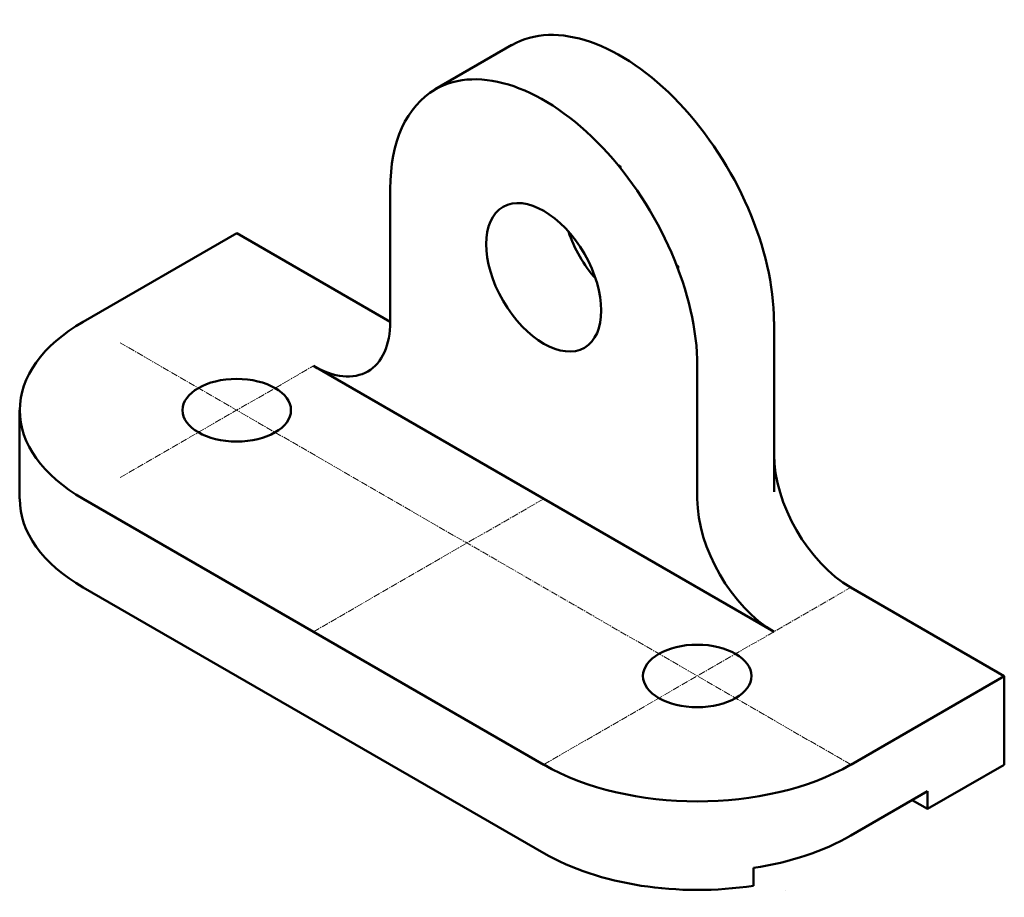
# Model space of a CAD drawing. Units: millimetres. Extents: x -15 to 96, y 7 to 106.
import ezdxf

# ---------------------------------------------------------------- set-up
doc = ezdxf.new("R2010")
doc.units = ezdxf.units.MM
doc.header["$MEASUREMENT"] = 0
doc.linetypes.add('CENTER2', pattern=[1.125, 0.75, -0.125, 0.125, -0.125])
doc.layers.add('M-CNTR', color=1, linetype='CENTER2', lineweight=18)
doc.layers.add('M-OUTL', color=7, linetype='Continuous', lineweight=50)

msp = doc.modelspace()

# ---------------------------------------------------------------- linework, layer by layer
at = {"layer": 'M-CNTR'}
for p, q in [((78.96, 21.51), (-3.47, 69.1)), ((-3.47, 53.92), (18.33, 66.51)), ((18.33, 36.51), (44.31, 51.51)), ((44.31, 21.51), (79.06, 41.57))]:
    msp.add_line(p, q, dxfattribs=at)
at = {"layer": 'M-OUTL'}
for p, q in [((40.73, 102.73), (32.07, 97.73)), ((27, 71.5), (27, 86.5)), ((-7.64, 71.5), (9.68, 81.5)), ((27, 71.5), (9.68, 81.5)), ((70.3, 71.51), (70.3, 52.29)), ((70.3, 36.5), (18.34, 66.5)), ((61.64, 66.5), (61.64, 51.5)), ((-14.82, 51.5), (-14.82, 61.5)), ((44.32, 21.5), (-7.64, 51.5)), ((44.32, 11.5), (-7.64, 41.5)), ((96.28, 31.5), (78.96, 41.5)), ((78.96, 21.5), (96.28, 31.5)), ((96.28, 21.5), (96.28, 31.5)), ((87.62, 16.5), (96.28, 21.5)), ((78.96, 13.5), (87.62, 18.5)), ((87.62, 16.5), (87.62, 18.5)), ((87.62, 16.5), (85.89, 17.5)), ((67.98, 7.84), (67.98, 9.84))]:
    msp.add_line(p, q, dxfattribs=at)
msp.add_lwpolyline([(71.63, 7.29), (71.63, 7.29)], close=True, dxfattribs=at)
for centre, major_axis, start_param, end_param in [((52.97, 81.51), (12.25, -21.21), 7.068583, 9.424778), ((44.32, 76.5), (12.25, -21.21), 0.785398, 3.141593), ((44.32, 76.5), (12.25, -21.21), 3.141593, 3.926991), ((52.97, 81.51), (4.59, -7.95), 4.372552, 5.052226), ((9.68, 61.5), (-24.49, 0), 5.497787, 6.283185), ((18.34, 76.5), (-6.12, 10.61), 3.141593, 3.926968), ((18.34, 76.5), (-6.12, 10.61), 2.356218, 3.141593), ((9.68, 61.5), (-24.49, 0), 0, 0.785398), ((78.96, 51.5), (-6.12, 10.61), 0.785421, 2.356171), ((9.68, 51.5), (-24.49, 0), 0, 0.785398), ((70.3, 46.5), (-6.12, 10.61), 0.785421, 2.356171), ((61.64, 31.5), (24.49, 0), 3.926991, 5.497787), ((61.64, 23.5), (24.49, 0), 4.974188, 5.497787), ((61.64, 21.5), (24.49, 0), 3.926991, 4.974188)]:
    msp.add_ellipse(centre, major_axis=major_axis, ratio=0.57735, start_param=start_param, end_param=end_param, dxfattribs=at)
for centre, major_axis in [((44.31, 76.51), (4.59, -7.95)), ((9.67, 61.51), (-6.12, 0)), ((61.63, 31.51), (-6.12, 0))]:
    msp.add_ellipse(centre, major_axis=major_axis, ratio=0.57735, dxfattribs=at)
for points, weights, knots in [([(52.97, 88.83), (52.97, 88.92), (52.97, 89.01), (52.84, 89.09), (52.71, 89.16)], [1, 1, 1, 0.999791477992, 1], [0, 0, 0, 1, 1, 1.040844, 1.040844, 1.040844]), ([(59.46, 77.46), (59.47, 77.61), (59.47, 77.76), (59.39, 77.81), (59.31, 77.85)], [1, 0.999791477992, 1, 1, 1], [0, 0, 0, 0.040844, 0.040844, 1.040844, 1.040844, 1.040844])]:
    msp.add_rational_spline(points, weights, degree=2, knots=knots, dxfattribs=at)

doc.saveas('drawing.dxf')
